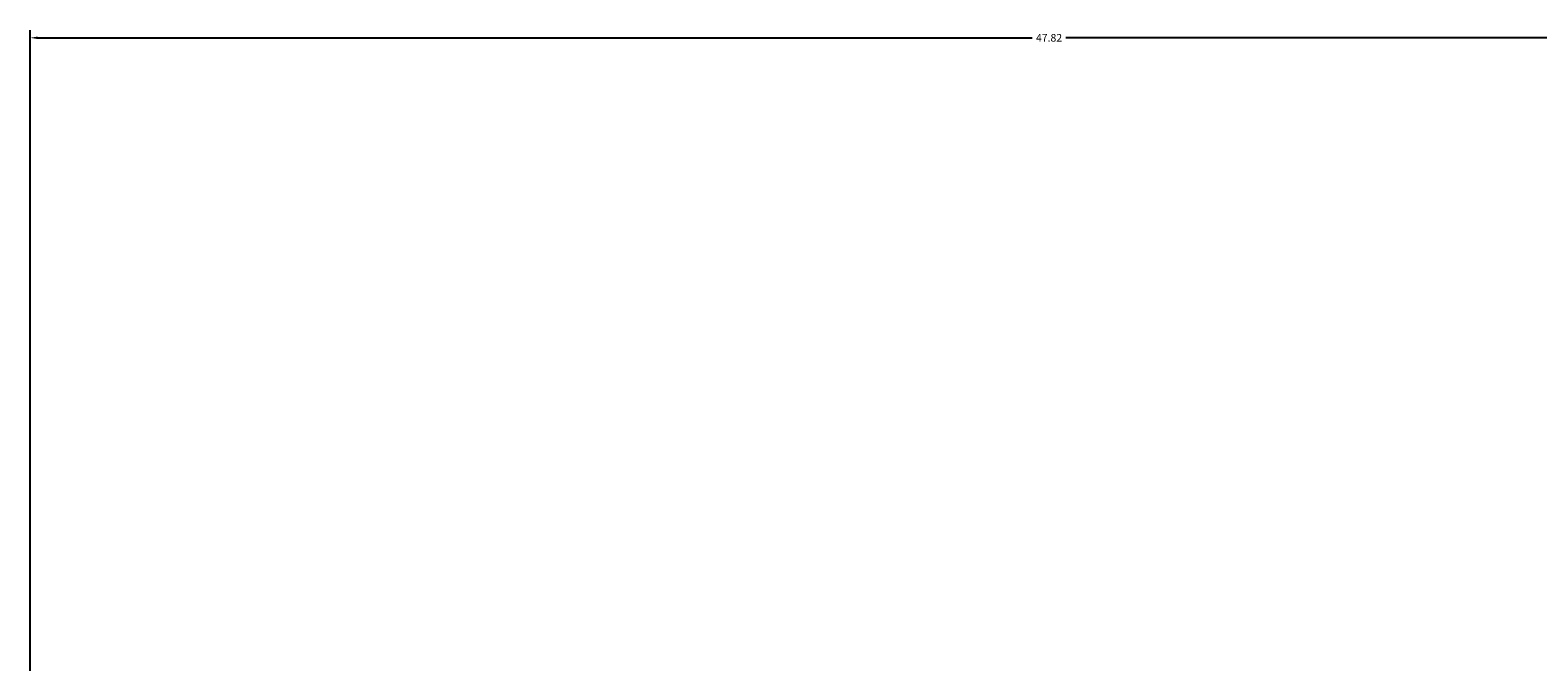
# Model space of a CAD drawing. Units: millimetres. Extents: x -11 to 280, y -4 to 208.
# Tile 17 of 55: x 31 to 66, y 193 to 208. Entities that reach past the tile are written whole.
import ezdxf

# ---------------------------------------------------------------- set-up
doc = ezdxf.new("R2010")
doc.units = ezdxf.units.MM
doc.layers.add('M-DIMS', color=2, linetype='Continuous', lineweight=18)
doc.styles.get("Standard").update_dxf_attribs({"font": 'arial.ttf'})
doc.dimstyles.get("Standard").update_dxf_attribs({"dimtxt": 0.18, "dimasz": 0.18, "dimexe": 0.18, "dimexo": 0.0625, "dimgap": 0.09, "dimtad": 0, "dimtih": 1, "dimtoh": 1, "dimdec": 4, "dimzin": 0, "dimdsep": 46, "dimtxsty": 'Standard', "dimcen": 0.09, "dimadec": 0, "dimazin": 0, "dimtfac": 1, "dimtdec": 4, "dimtofl": 0, "dimtmove": 0, "dimatfit": 3, "dimfxl": 1, "dimtolj": 1, "dimtzin": 0, "dimarcsym": 0})

# ---------------------------------------------------------------- blocks, each defined once
blk = doc.blocks.new('*D9')
at = {"layer": 'Defpoints', "color": 0, "transparency": 16777216}
for p in [(78.827, 207.495), (31.006, 98.021), (78.827, 98.149)]:
    blk.add_point(p, dxfattribs=at)
at = {"layer": 'M-DIMS', "color": 0, "lineweight": -2, "transparency": 16777216}
for p, q in [((31.006, 98.084), (31.006, 207.675)), ((31.186, 207.495), (54.52, 207.495)), ((78.647, 207.495), (55.313, 207.495)), ((78.827, 98.212), (78.827, 207.675))]:
    blk.add_line(p, q, dxfattribs=at)
at = {"layer": 'M-DIMS', "color": 0, "transparency": 16777216}
for points in [[(31.186, 207.525), (31.186, 207.465), (31.006, 207.495)], [(78.647, 207.525), (78.647, 207.465), (78.827, 207.495)]]:
    blk.add_solid(points, dxfattribs=at)
at = {"layer": 'M-DIMS', "color": 0, "transparency": 16777216, "insert": (54.917, 207.495), "char_height": 0.18, "attachment_point": 5}
blk.add_mtext('\\A1;47.82', dxfattribs=at)

msp = doc.modelspace()

# ---------------------------------------------------------------- dimensions: what is measured, and where the dimension line sits
at = {"layer": 'M-DIMS'}
dim = msp.add_linear_dim(base=(78.8273, 207.495), p1=(31.0059, 98.0213), p2=(78.8273, 98.1491), dimstyle='Standard', override={"dimdec": 2, "dimlfac": 1, "dimrnd": 0, "dimzin": 0, "dimdsep": 46, "dimlunit": 2}, dxfattribs=at)
dim.commit()
dim.dimension.update_dxf_attribs({"geometry": '*D9', "text_midpoint": (54.9166, 207.495)})

doc.saveas('drawing.dxf')
